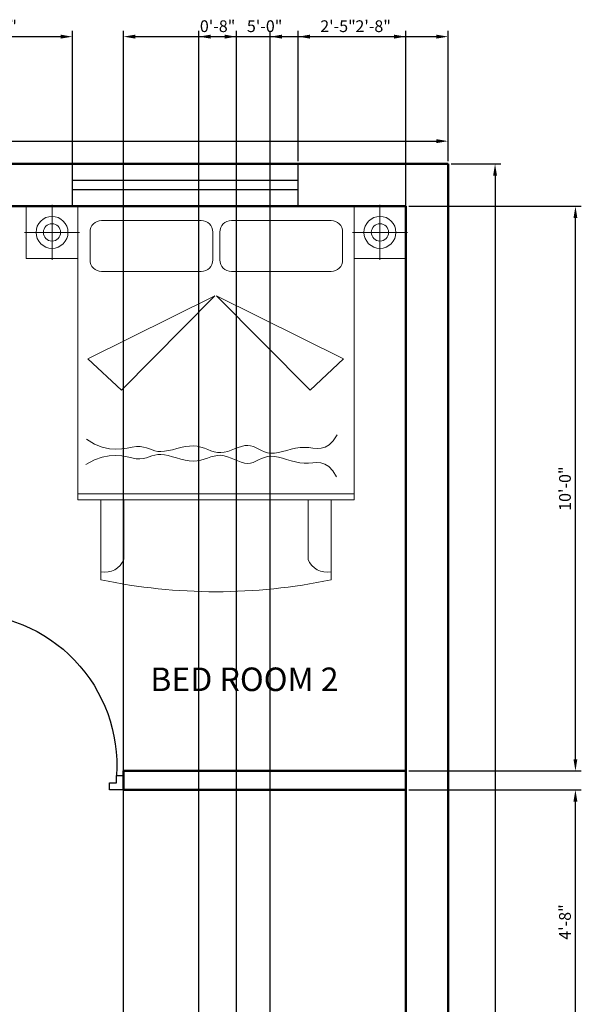
# Model space of a CAD drawing. Units: inches. Extents: x 1905 to 2315, y 3232 to 3824.
# Tile 8 of 8: x 2195 to 2314, y 3615 to 3824. Entities that reach past the tile are written whole.
import ezdxf

# ---------------------------------------------------------------- set-up
doc = ezdxf.new("R2010")
doc.units = ezdxf.units.IN
for name, color, linetype, lineweight in [('A-ANNO-DIMS', 2, 'Continuous', 18), ('A-AREA-IDEN', 7, 'Continuous', 25), ('A-FURN', 8, 'Continuous', 18), ('door', 1, 'Continuous', 25), ('wall', 2, 'Continuous', 50), ('WINDOW', 60, 'Continuous', 25)]:
    doc.layers.add(name, color=color, linetype=linetype, lineweight=lineweight)
doc.styles.get("Standard").update_dxf_attribs({"font": 'arial.ttf'})
doc.dimstyles.new('ISO-25', dxfattribs={"dimtxt": 2.5, "dimasz": 2.5, "dimexe": 1.25, "dimexo": 0.625, "dimtad": 1, "dimdec": 1, "dimlunit": 3, "dimtxsty": 'Standard', "dimcen": 2.5, "dimadec": 0, "dimazin": 0, "dimtfac": 1, "dimtdec": 1, "dimtmove": 0, "dimatfit": 3, "dimfxl": 1, "dimarcsym": 0})

# ---------------------------------------------------------------- blocks, each defined once
blk = doc.blocks.new('A$C4F543DC7')
for p, q in [((0.0134, 3.35, -0.1688), (3.3134, 3.35, -0.1688)), ((0.4634, 3.35, -0.1688), (0.0134, 3.35, -0.1688)), ((0.0134, 2.896, -0.1688), (0.0134, 3.35, -0.1688)), ((0.0134, 3.35, -0.1688), (0.0134, 2.896, -0.1688)), ((0.2381, 3.1233, -0.4388), (0.2381, 3.3614, -0.4388)), ((0.4634, 3.35, -0.1688), (0.4634, 0.8, -0.1688)), ((2.8634, 3.35, -0.1688), (0.4634, 3.35, -0.1688)), ((0.4634, 2.896, -0.1688), (0.4634, 3.35, -0.1688)), ((2.8634, 0.8, -0.1688), (2.8634, 3.35, -0.1688)), ((2.8634, 3.35, -0.1688), (3.3134, 3.35, -0.1688)), ((2.8634, 2.896, -0.1688), (2.8634, 3.35, -0.1688)), ((3.0888, 3.1233, -0.4388), (3.0888, 3.3614, -0.4388)), ((3.3134, 3.35, -0.1688), (3.3134, 2.896, -0.1688)), ((3.3134, 3.35, -0.1688), (3.3134, 2.896, -0.1688)), ((1.5354, 3.226, -0.1688), (0.6684, 3.226, -0.1688)), ((2.6644, 3.226, -0.1688), (1.7974, 3.226, -0.1688)), ((0.2381, 3.1233, -0.4388), (0, 3.1233, -0.4388)), ((0.2381, 3.1233, -0.4388), (0.4762, 3.1233, -0.4388)), ((0.2381, 3.1233, -0.4388), (0.2381, 2.8852, -0.4388)), ((0.5684, 3.126, -0.1688), (0.5684, 2.884, -0.1688)), ((1.6354, 2.884, -0.1688), (1.6354, 3.126, -0.1688)), ((1.6974, 3.126, -0.1688), (1.6974, 2.884, -0.1688)), ((2.7644, 2.884, -0.1688), (2.7644, 3.126, -0.1688)), ((3.0888, 3.1233, -0.4388), (2.8507, 3.1233, -0.4388)), ((3.0888, 3.1233, -0.4388), (3.0888, 2.8852, -0.4388)), ((3.0888, 3.1233, -0.4388), (3.3269, 3.1233, -0.4388)), ((0.4634, 2.896, -0.1688), (0.0134, 2.896, -0.1688)), ((0.0134, 2.896, -0.1688), (0.4634, 2.896, -0.1688)), ((0.4634, 0.8, -0.1688), (0.4634, 2.896, -0.1688)), ((2.8634, 2.896, -0.1688), (2.8634, 0.8, -0.1688)), ((3.3134, 2.896, -0.1688), (2.8634, 2.896, -0.1688)), ((3.3134, 2.896, -0.1688), (2.8634, 2.896, -0.1688)), ((0.6684, 2.784, -0.1688), (1.5354, 2.784, -0.1688)), ((1.7974, 2.784, -0.1688), (2.6644, 2.784, -0.1688)), ((1.6534, 2.573, -0.1688), (0.5504, 2.025, -0.1688)), ((0.8414, 1.752, -0.1688), (1.6534, 2.573, -0.1688)), ((2.4814, 1.752, -0.1688), (1.6694, 2.573, -0.1688)), ((1.6694, 2.573, -0.1688), (2.7724, 2.025, -0.1688)), ((0.5504, 2.025, -0.1688), (0.8414, 1.752, -0.1688)), ((2.7724, 2.025, -0.1688), (2.4814, 1.752, -0.1688)), ((0.5369, 1.3267, -0.1688), (0.6088, 1.2835, -0.1688)), ((2.6479, 1.2774, -0.1688), (2.683, 1.312, -0.1688)), ((2.683, 1.312, -0.1688), (2.7182, 1.3641, -0.1688)), ((0.6088, 1.2835, -0.1688), (0.6756, 1.2566, -0.1688)), ((0.6756, 1.2566, -0.1688), (0.7373, 1.2428, -0.1688)), ((0.7373, 1.2428, -0.1688), (0.794, 1.239, -0.1688)), ((0.794, 1.239, -0.1688), (0.8457, 1.242, -0.1688)), ((0.8457, 1.242, -0.1688), (0.8925, 1.2489, -0.1688)), ((0.8925, 1.2489, -0.1688), (0.9345, 1.2564, -0.1688)), ((0.9345, 1.2564, -0.1688), (0.9718, 1.2615, -0.1688)), ((0.9718, 1.2615, -0.1688), (1.0044, 1.2617, -0.1688)), ((1.0044, 1.2617, -0.1688), (1.0334, 1.2578, -0.1688)), ((1.0334, 1.2578, -0.1688), (1.0597, 1.2509, -0.1688)), ((1.0597, 1.2509, -0.1688), (1.0842, 1.2424, -0.1688)), ((1.0842, 1.2424, -0.1688), (1.1081, 1.2336, -0.1688)), ((1.1081, 1.2336, -0.1688), (1.1322, 1.2257, -0.1688)), ((1.1322, 1.2257, -0.1688), (1.1577, 1.2201, -0.1688)), ((1.1577, 1.2201, -0.1688), (1.1855, 1.218, -0.1688)), ((1.1855, 1.218, -0.1688), (1.2163, 1.2204, -0.1688)), ((1.2163, 1.2204, -0.1688), (1.2498, 1.2264, -0.1688)), ((1.2498, 1.2264, -0.1688), (1.2852, 1.2347, -0.1688)), ((1.2852, 1.2347, -0.1688), (1.3218, 1.2441, -0.1688)), ((1.3218, 1.2441, -0.1688), (1.3591, 1.2533, -0.1688)), ((1.3591, 1.2533, -0.1688), (1.3963, 1.2612, -0.1688)), ((1.3963, 1.2612, -0.1688), (1.4328, 1.2664, -0.1688)), ((1.4328, 1.2664, -0.1688), (1.4679, 1.2677, -0.1688)), ((1.4679, 1.2677, -0.1688), (1.501, 1.2643, -0.1688)), ((1.501, 1.2643, -0.1688), (1.5324, 1.257, -0.1688)), ((1.5324, 1.257, -0.1688), (1.5624, 1.2473, -0.1688)), ((1.5624, 1.2473, -0.1688), (1.5915, 1.2365, -0.1688)), ((1.5915, 1.2365, -0.1688), (1.6199, 1.2259, -0.1688)), ((1.6199, 1.2259, -0.1688), (1.6481, 1.2169, -0.1688)), ((1.6481, 1.2169, -0.1688), (1.6765, 1.2108, -0.1688)), ((1.6765, 1.2108, -0.1688), (1.7053, 1.209, -0.1688)), ((1.7053, 1.209, -0.1688), (1.7349, 1.2124, -0.1688)), ((1.7349, 1.2124, -0.1688), (1.7651, 1.2199, -0.1688)), ((1.7651, 1.2199, -0.1688), (1.7955, 1.2301, -0.1688)), ((1.7955, 1.2301, -0.1688), (1.8258, 1.2417, -0.1688)), ((1.8258, 1.2417, -0.1688), (1.8557, 1.2531, -0.1688)), ((1.8557, 1.2531, -0.1688), (1.8849, 1.263, -0.1688)), ((1.8849, 1.263, -0.1688), (1.913, 1.2698, -0.1688)), ((1.913, 1.2698, -0.1688), (1.9397, 1.2722, -0.1688)), ((1.9397, 1.2722, -0.1688), (1.9649, 1.2692, -0.1688)), ((1.9649, 1.2692, -0.1688), (1.989, 1.2617, -0.1688)), ((1.989, 1.2617, -0.1688), (2.0124, 1.2512, -0.1688)), ((2.0124, 1.2512, -0.1688), (2.0359, 1.2391, -0.1688)), ((2.0359, 1.2391, -0.1688), (2.0599, 1.2269, -0.1688)), ((2.0599, 1.2269, -0.1688), (2.0849, 1.216, -0.1688)), ((2.0849, 1.216, -0.1688), (2.1117, 1.2077, -0.1688)), ((2.1117, 1.2077, -0.1688), (2.1407, 1.2037, -0.1688)), ((2.1407, 1.2037, -0.1688), (2.1723, 1.2047, -0.1688)), ((2.1723, 1.2047, -0.1688), (2.2062, 1.21, -0.1688)), ((2.2062, 1.21, -0.1688), (2.242, 1.2182, -0.1688)), ((2.242, 1.2182, -0.1688), (2.2791, 1.2279, -0.1688)), ((2.2791, 1.2279, -0.1688), (2.3173, 1.2378, -0.1688)), ((2.3173, 1.2378, -0.1688), (2.3558, 1.2465, -0.1688)), ((2.3558, 1.2465, -0.1688), (2.3944, 1.2527, -0.1688)), ((2.3944, 1.2527, -0.1688), (2.4325, 1.255, -0.1688)), ((2.4325, 1.255, -0.1688), (2.4698, 1.2529, -0.1688)), ((2.4698, 1.2529, -0.1688), (2.5064, 1.2488, -0.1688)), ((2.5064, 1.2488, -0.1688), (2.5423, 1.2459, -0.1688)), ((2.5423, 1.2459, -0.1688), (2.5777, 1.2476, -0.1688)), ((2.5777, 1.2476, -0.1688), (2.6129, 1.257, -0.1688)), ((2.6129, 1.257, -0.1688), (2.6479, 1.2774, -0.1688)), ((0.5334, 1.105, -0.1688), (0.6067, 1.1458, -0.1688)), ((0.6067, 1.1458, -0.1688), (0.6743, 1.1706, -0.1688)), ((0.6743, 1.1706, -0.1688), (0.7364, 1.1825, -0.1688)), ((0.7364, 1.1825, -0.1688), (0.7931, 1.1846, -0.1688)), ((0.7931, 1.1846, -0.1688), (0.8447, 1.1799, -0.1688)), ((0.8447, 1.1799, -0.1688), (0.8913, 1.1716, -0.1688)), ((0.8913, 1.1716, -0.1688), (0.9331, 1.1628, -0.1688)), ((0.9331, 1.1628, -0.1688), (0.9701, 1.1565, -0.1688)), ((0.9701, 1.1565, -0.1688), (1.0027, 1.1552, -0.1688)), ((1.0027, 1.1552, -0.1688), (1.0318, 1.1582, -0.1688)), ((1.0318, 1.1582, -0.1688), (1.0583, 1.1642, -0.1688)), ((1.0583, 1.1642, -0.1688), (1.0831, 1.172, -0.1688)), ((1.0831, 1.172, -0.1688), (1.1072, 1.18, -0.1688)), ((1.1072, 1.18, -0.1688), (1.1316, 1.1872, -0.1688)), ((1.1316, 1.1872, -0.1688), (1.1573, 1.192, -0.1688)), ((1.1573, 1.192, -0.1688), (1.1851, 1.1932, -0.1688)), ((1.1851, 1.1932, -0.1688), (1.2158, 1.1898, -0.1688)), ((1.2158, 1.1898, -0.1688), (1.2491, 1.1828, -0.1688)), ((1.2491, 1.1828, -0.1688), (1.2842, 1.1734, -0.1688)), ((1.2842, 1.1734, -0.1688), (1.3206, 1.1629, -0.1688)), ((1.3206, 1.1629, -0.1688), (1.3575, 1.1524, -0.1688)), ((1.3575, 1.1524, -0.1688), (1.3945, 1.1434, -0.1688)), ((1.3945, 1.1434, -0.1688), (1.4308, 1.1371, -0.1688)), ((1.4308, 1.1371, -0.1688), (1.4658, 1.1347, -0.1688)), ((1.4658, 1.1347, -0.1688), (1.499, 1.137, -0.1688)), ((1.499, 1.137, -0.1688), (1.5306, 1.1433, -0.1688)), ((1.5306, 1.1433, -0.1688), (1.5609, 1.152, -0.1688)), ((1.5609, 1.152, -0.1688), (1.5903, 1.1619, -0.1688)), ((1.5903, 1.1619, -0.1688), (1.6191, 1.1716, -0.1688)), ((1.6191, 1.1716, -0.1688), (1.6475, 1.1797, -0.1688)), ((1.6475, 1.1797, -0.1688), (1.676, 1.1849, -0.1688)), ((1.676, 1.1849, -0.1688), (1.7049, 1.1858, -0.1688)), ((1.7049, 1.1858, -0.1688), (1.7344, 1.1816, -0.1688)), ((1.7344, 1.1816, -0.1688), (1.7643, 1.1731, -0.1688)), ((1.7643, 1.1731, -0.1688), (1.7944, 1.1619, -0.1688)), ((1.7944, 1.1619, -0.1688), (1.8244, 1.1494, -0.1688)), ((1.8244, 1.1494, -0.1688), (1.8539, 1.137, -0.1688)), ((1.8539, 1.137, -0.1688), (1.8827, 1.1263, -0.1688)), ((1.8827, 1.1263, -0.1688), (1.9106, 1.1186, -0.1688)), ((1.9106, 1.1186, -0.1688), (1.9373, 1.1153, -0.1688)), ((1.9373, 1.1153, -0.1688), (1.9625, 1.1176, -0.1688)), ((1.9625, 1.1176, -0.1688), (1.9868, 1.1243, -0.1688)), ((1.9868, 1.1243, -0.1688), (2.0106, 1.134, -0.1688)), ((2.0106, 1.134, -0.1688), (2.0344, 1.1454, -0.1688)), ((2.0344, 1.1454, -0.1688), (2.0588, 1.1568, -0.1688)), ((2.0588, 1.1568, -0.1688), (2.0842, 1.167, -0.1688)), ((2.0842, 1.167, -0.1688), (2.1112, 1.1743, -0.1688)), ((2.1112, 1.1743, -0.1688), (2.1403, 1.1775, -0.1688)), ((2.1403, 1.1775, -0.1688), (2.1718, 1.1755, -0.1688)), ((2.1718, 1.1755, -0.1688), (2.2056, 1.1691, -0.1688)), ((2.2056, 1.1691, -0.1688), (2.2411, 1.1598, -0.1688)), ((2.2411, 1.1598, -0.1688), (2.2779, 1.1489, -0.1688)), ((2.2779, 1.1489, -0.1688), (2.3157, 1.1379, -0.1688)), ((2.3157, 1.1379, -0.1688), (2.354, 1.1279, -0.1688)), ((2.354, 1.1279, -0.1688), (2.3923, 1.1205, -0.1688)), ((2.3923, 1.1205, -0.1688), (2.4304, 1.117, -0.1688)), ((2.4304, 1.117, -0.1688), (2.4677, 1.118, -0.1688)), ((2.4677, 1.118, -0.1688), (2.5043, 1.1209, -0.1688)), ((2.5043, 1.1209, -0.1688), (2.5403, 1.1226, -0.1688)), ((2.5403, 1.1226, -0.1688), (2.5757, 1.1199, -0.1688)), ((2.5757, 1.1199, -0.1688), (2.6106, 1.1094, -0.1688)), ((2.6106, 1.1094, -0.1688), (2.645, 1.0879, -0.1688)), ((2.645, 1.0879, -0.1688), (2.6789, 1.0522, -0.1688)), ((2.6789, 1.0522, -0.1688), (2.7124, 0.999, -0.1688)), ((0.4634, 0.85, -0.1688), (2.8634, 0.85, -0.1688)), ((0.4634, 0.8, -0.1688), (2.8634, 0.8, -0.1688)), ((0.6634, 0.8, -0.1688), (0.4634, 0.8, -0.1688)), ((0.6634, 0.8, -0.1688), (2.6634, 0.8, -0.1688)), ((0.6634, 0.104, -0.1688), (0.6634, 0.8, -0.1688)), ((0.6634, 0.104, -0.1688), (0.6634, 0.8, -0.1688)), ((0.8634, 0.281, -0.1688), (0.8634, 0.8, -0.1688)), ((2.4634, 0.8, -0.1688), (2.4634, 0.281, -0.1688)), ((2.8634, 0.8, -0.1688), (2.6634, 0.8, -0.1688)), ((2.6634, 0.8, -0.1688), (2.6634, 0.104, -0.1688)), ((2.6634, 0.8, -0.1688), (2.6634, 0.104, -0.1688))]:
    blk.add_line(p, q)
for centre, radius in [((0.2381, 3.1233, -0.4388), 0.139), ((3.0888, 3.1233, -0.4388), 0.139), ((0.2381, 3.1233, -0.4388), 0.075), ((3.0888, 3.1233, -0.4388), 0.075)]:
    blk.add_circle(centre, radius)
for centre, radius, start, end in [((0.6684, 3.126, -0.1688), 0.1, 90, 180), ((1.5354, 3.126, -0.1688), 0.1, 0, 90), ((1.7974, 3.126, -0.1688), 0.1, 90, 180), ((2.6644, 3.126, -0.1688), 0.1, 0, 90), ((0.6684, 2.884, -0.1688), 0.1, 180, 270), ((1.5354, 2.884, -0.1688), 0.1, 270, 0), ((1.7974, 2.884, -0.1688), 0.1, 180, 270), ((2.6644, 2.884, -0.1688), 0.1, 270, 0), ((0.6994, 0.3472, -0.1688), 0.1769, 258.2616, 338.03196), ((2.6275, 0.3472, -0.1688), 0.1769, 201.96804, 281.7384), ((1.6634, 4.8597, -0.1688), 4.8597, 258.12517, 281.87483), ((1.6634, 4.8597, -0.1688), 4.8597, 258.12517, 281.87483)]:
    blk.add_arc(centre, radius, start, end)
blk = doc.blocks.new('*D15')
at = {"layer": 'A-ANNO-DIMS', "color": 0, "lineweight": -2, "transparency": 16777216}
for p, q in [((1938.01, 3793.86), (1938.01, 3799.33)), ((2286.01, 3793.86), (2286.01, 3799.33)), ((1940.51, 3798.08), (2283.51, 3798.08))]:
    blk.add_line(p, q, dxfattribs=at)
at = {"layer": 'A-ANNO-DIMS', "color": 0, "transparency": 16777216}
for points in [[(1940.51, 3798.5), (1940.51, 3797.67), (1938.01, 3798.08)], [(2283.51, 3798.5), (2283.51, 3797.67), (2286.01, 3798.08)]]:
    blk.add_solid(points, dxfattribs=at)
at = {"layer": 'Defpoints', "color": 0, "transparency": 16777216}
for p in [(2286.01, 3798.08), (1938.01, 3793.23), (2286.01, 3793.23)]:
    blk.add_point(p, dxfattribs=at)
at = {"layer": 'A-ANNO-DIMS', "color": 0, "transparency": 16777216, "insert": (2112.01, 3799.99), "char_height": 2.5, "attachment_point": 5}
blk.add_mtext("29'", dxfattribs=at)
blk = doc.blocks.new('*D16')
at = {"layer": 'A-ANNO-DIMS', "color": 0, "lineweight": -2, "transparency": 16777216}
for p, q in [((2286.63, 3793.23), (2297.23, 3793.23)), ((2295.98, 3790.73), (2295.98, 3279.73)), ((2286.63, 3277.23), (2297.23, 3277.23))]:
    blk.add_line(p, q, dxfattribs=at)
at = {"layer": 'A-ANNO-DIMS', "color": 0, "transparency": 16777216}
for points in [[(2295.57, 3790.73), (2296.4, 3790.73), (2295.98, 3793.23)], [(2295.57, 3279.73), (2296.4, 3279.73), (2295.98, 3277.23)]]:
    blk.add_solid(points, dxfattribs=at)
at = {"layer": 'Defpoints', "color": 0, "transparency": 16777216}
for p in [(2286.01, 3793.23), (2286.01, 3277.23), (2295.98, 3277.23)]:
    blk.add_point(p, dxfattribs=at)
at = {"layer": 'A-ANNO-DIMS', "color": 0, "transparency": 16777216, "insert": (2294.08, 3535.23), "char_height": 2.5, "attachment_point": 5, "rotation": 90}
blk.add_mtext("43'", dxfattribs=at)
blk = doc.blocks.new('DOOR-SWING-36IN')
for p, q in [((34.51, 36), (37.51, 36)), ((34.51, 34.5), (34.51, 36)), ((37.51, 36), (37.51, 33)), ((36.01, 34.5), (0.01, 34.5)), ((36.01, 34.5), (34.51, 34.5)), ((36.01, 33), (36.01, 34.5)), ((36.01, 33), (0.01, 33)), ((37.51, 33), (36.01, 33)), ((37.51, 3), (36.01, 3)), ((36.01, 3), (36.01, 1.5)), ((37.51, 0), (37.51, 3)), ((36.01, 1.5), (34.51, 1.5)), ((34.51, 1.5), (34.51, 0)), ((34.51, 0), (37.51, 0))]:
    blk.add_line(p, q)
blk.add_arc((32.32, 33.75), 32.32, 178.6705, 273.8756)
blk = doc.blocks.new('WIN-48IN')
for p, q in [((0, 9), (0, 0)), ((0, 9), (48, 9)), ((48, 9), (48, 0)), ((0, 5.5), (48, 5.5)), ((0, 3.5), (48, 3.5)), ((0, 0), (48, 0))]:
    blk.add_line(p, q)
blk = doc.blocks.new('*D42')
at = {"layer": 'A-ANNO-DIMS', "color": 0, "lineweight": -2, "transparency": 16777216}
for p, q in [((2175.01, 3784.86), (2175.01, 3821.54)), ((2206.15, 3784.86), (2206.15, 3821.54)), ((2177.51, 3820.29), (2203.65, 3820.29))]:
    blk.add_line(p, q, dxfattribs=at)
at = {"layer": 'A-ANNO-DIMS', "color": 0, "transparency": 16777216}
for points in [[(2177.51, 3820.71), (2177.51, 3819.88), (2175.01, 3820.29)], [(2203.65, 3820.71), (2203.65, 3819.88), (2206.15, 3820.29)]]:
    blk.add_solid(points, dxfattribs=at)
at = {"layer": 'Defpoints', "color": 0, "transparency": 16777216}
for p in [(2206.15, 3820.29), (2175.01, 3784.23), (2206.15, 3784.23)]:
    blk.add_point(p, dxfattribs=at)
at = {"layer": 'A-ANNO-DIMS', "color": 0, "transparency": 16777216, "insert": (2190.58, 3822.17), "char_height": 2.5, "attachment_point": 5}
blk.add_mtext('2\'-7"', dxfattribs=at)
blk = doc.blocks.new('*D43')
at = {"layer": 'A-ANNO-DIMS', "color": 0, "lineweight": -2, "transparency": 16777216}
for p, q in [((2254.15, 3793.86), (2254.15, 3821.54)), ((2286.01, 3793.86), (2286.01, 3821.54)), ((2256.65, 3820.29), (2283.51, 3820.29))]:
    blk.add_line(p, q, dxfattribs=at)
at = {"layer": 'A-ANNO-DIMS', "color": 0, "transparency": 16777216}
for points in [[(2256.65, 3820.71), (2256.65, 3819.88), (2254.15, 3820.29)], [(2283.51, 3820.71), (2283.51, 3819.88), (2286.01, 3820.29)]]:
    blk.add_solid(points, dxfattribs=at)
at = {"layer": 'Defpoints', "color": 0, "transparency": 16777216}
for p in [(2286.01, 3820.29), (2254.15, 3793.23), (2286.01, 3793.23)]:
    blk.add_point(p, dxfattribs=at)
at = {"layer": 'A-ANNO-DIMS', "color": 0, "transparency": 16777216, "insert": (2270.08, 3822.19), "char_height": 2.5, "attachment_point": 5}
blk.add_mtext('2\'-8"', dxfattribs=at)
blk = doc.blocks.new('*D54')
at = {"layer": 'A-ANNO-DIMS', "color": 0, "lineweight": -2, "transparency": 16777216}
for p, q in [((2277.63, 3660.23), (2314.32, 3660.23)), ((2313.07, 3606.51), (2313.07, 3657.73)), ((2277.63, 3604.01), (2314.32, 3604.01))]:
    blk.add_line(p, q, dxfattribs=at)
at = {"layer": 'A-ANNO-DIMS', "color": 0, "transparency": 16777216}
for points in [[(2312.65, 3657.73), (2313.48, 3657.73), (2313.07, 3660.23)], [(2312.65, 3606.51), (2313.48, 3606.51), (2313.07, 3604.01)]]:
    blk.add_solid(points, dxfattribs=at)
at = {"layer": 'Defpoints', "color": 0, "transparency": 16777216}
for p in [(2277.01, 3660.23), (2313.07, 3660.23), (2277.01, 3604.01)]:
    blk.add_point(p, dxfattribs=at)
at = {"layer": 'A-ANNO-DIMS', "color": 0, "transparency": 16777216, "insert": (2311.17, 3632.12), "char_height": 2.5, "attachment_point": 5, "rotation": 90}
blk.add_mtext('4\'-8"', dxfattribs=at)
blk = doc.blocks.new('*D55')
at = {"layer": 'A-ANNO-DIMS', "color": 0, "lineweight": -2, "transparency": 16777216}
for p, q in [((2277.63, 3784.23), (2314.32, 3784.23)), ((2313.07, 3666.73), (2313.07, 3781.73)), ((2277.63, 3664.23), (2314.32, 3664.23))]:
    blk.add_line(p, q, dxfattribs=at)
at = {"layer": 'A-ANNO-DIMS', "color": 0, "transparency": 16777216}
for points in [[(2312.65, 3781.73), (2313.48, 3781.73), (2313.07, 3784.23)], [(2312.65, 3666.73), (2313.48, 3666.73), (2313.07, 3664.23)]]:
    blk.add_solid(points, dxfattribs=at)
at = {"layer": 'Defpoints', "color": 0, "transparency": 16777216}
for p in [(2277.01, 3784.23), (2313.07, 3784.23), (2277.01, 3664.23)]:
    blk.add_point(p, dxfattribs=at)
at = {"layer": 'A-ANNO-DIMS', "color": 0, "transparency": 16777216, "insert": (2311.17, 3724.23), "char_height": 2.5, "attachment_point": 5, "rotation": 90}
blk.add_mtext('10\'-0"', dxfattribs=at)
blk = doc.blocks.new('*D62')
at = {"layer": 'A-ANNO-DIMS', "color": 0, "lineweight": -2, "transparency": 16777216}
for p, q in [((2233.01, 3322.86), (2233.01, 3821.54)), ((2241.01, 3322.86), (2241.01, 3821.54)), ((2235.51, 3820.29), (2238.51, 3820.29))]:
    blk.add_line(p, q, dxfattribs=at)
at = {"layer": 'A-ANNO-DIMS', "color": 0, "transparency": 16777216}
for points in [[(2235.51, 3820.71), (2235.51, 3819.88), (2233.01, 3820.29)], [(2238.51, 3820.71), (2238.51, 3819.88), (2241.01, 3820.29)]]:
    blk.add_solid(points, dxfattribs=at)
at = {"layer": 'Defpoints', "color": 0, "transparency": 16777216}
for p in [(2241.01, 3820.29), (2233.01, 3322.23), (2241.01, 3322.23)]:
    blk.add_point(p, dxfattribs=at)
at = {"layer": 'A-ANNO-DIMS', "color": 0, "transparency": 16777216, "insert": (2237.01, 3822.19), "char_height": 2.5, "attachment_point": 5}
blk.add_mtext('0\'-8"', dxfattribs=at)
blk = doc.blocks.new('*D66')
at = {"layer": 'A-ANNO-DIMS', "color": 0, "lineweight": -2, "transparency": 16777216}
for p, q in [((2248.2, 3393.73), (2248.2, 3821.54)), ((2277.01, 3383.48), (2277.01, 3821.54)), ((2250.7, 3820.29), (2274.51, 3820.29))]:
    blk.add_line(p, q, dxfattribs=at)
at = {"layer": 'A-ANNO-DIMS', "color": 0, "transparency": 16777216}
for points in [[(2250.7, 3820.71), (2250.7, 3819.88), (2248.2, 3820.29)], [(2274.51, 3820.71), (2274.51, 3819.88), (2277.01, 3820.29)]]:
    blk.add_solid(points, dxfattribs=at)
at = {"layer": 'Defpoints', "color": 0, "transparency": 16777216}
for p in [(2277.01, 3820.29), (2248.2, 3393.11), (2277.01, 3382.85)]:
    blk.add_point(p, dxfattribs=at)
at = {"layer": 'A-ANNO-DIMS', "color": 0, "transparency": 16777216, "insert": (2262.6, 3822.19), "char_height": 2.5, "attachment_point": 5}
blk.add_mtext('2\'-5"', dxfattribs=at)
blk = doc.blocks.new('*D71')
at = {"layer": 'A-ANNO-DIMS', "color": 0, "lineweight": -2, "transparency": 16777216}
for p, q in [((2217.01, 3480.07), (2217.01, 3821.54)), ((2277.01, 3476.07), (2277.01, 3821.54)), ((2219.51, 3820.29), (2274.51, 3820.29))]:
    blk.add_line(p, q, dxfattribs=at)
at = {"layer": 'A-ANNO-DIMS', "color": 0, "transparency": 16777216}
for points in [[(2219.51, 3820.71), (2219.51, 3819.88), (2217.01, 3820.29)], [(2274.51, 3820.71), (2274.51, 3819.88), (2277.01, 3820.29)]]:
    blk.add_solid(points, dxfattribs=at)
at = {"layer": 'Defpoints', "color": 0, "transparency": 16777216}
for p in [(2277.01, 3820.29), (2217.01, 3479.45), (2277.01, 3475.45)]:
    blk.add_point(p, dxfattribs=at)
at = {"layer": 'A-ANNO-DIMS', "color": 0, "transparency": 16777216, "insert": (2247.01, 3822.19), "char_height": 2.5, "attachment_point": 5}
blk.add_mtext('5\'-0"', dxfattribs=at)

msp = doc.modelspace()

# ---------------------------------------------------------------- linework, layer by layer
at = {"layer": 'wall'}
for p, q in [((2286.01, 3793.23), (1938.01, 3793.23)), ((2286.01, 3277.23), (2286.01, 3793.23)), ((2277.01, 3784.23), (1947.01, 3784.23)), ((2277.01, 3286.23), (2277.01, 3784.23)), ((2277.01, 3664.23), (2217.01, 3664.23)), ((2217.01, 3664.23), (2217.01, 3660.23)), ((2277.01, 3660.23), (2217.01, 3660.23))]:
    msp.add_line(p, q, dxfattribs=at)

# ---------------------------------------------------------------- block references
at = {"layer": 'A-FURN', "xscale": 24.45263891714, "yscale": 24.45263891714, "zscale": 24.45263891714}
msp.add_blockref('A$C4F543DC7', (2195.99, 3702.32, 4.13), dxfattribs=at)
at = {"layer": 'door', "extrusion": (0, 0, -1), "zscale": -1, "rotation": 270.0000000000044}
msp.add_blockref('DOOR-SWING-36IN', (-2217.01, 3697.74), dxfattribs=at)
at = {"layer": 'WINDOW', "rotation": 180}
msp.add_blockref('WIN-48IN', (2254.15, 3793.23), dxfattribs=at)

# ---------------------------------------------------------------- texts
at = {"layer": 'A-AREA-IDEN', "insert": (2222.7, 3686.21), "char_height": 5, "attachment_point": 1}
msp.add_mtext_dynamic_manual_height_columns('BED ROOM 2', width=56.1502, gutter_width=12.5, heights=[0], dxfattribs=at)

# ---------------------------------------------------------------- dimensions: what is measured, and where the dimension line sits
at = {"layer": 'A-ANNO-DIMS'}
for base, p1, p2, override, picture, middle in [((2206.15, 3820.29), (2175.01, 3784.23), (2206.15, 3784.23), {"dimdec": 1, "dimlfac": 1, "dimrnd": 0, "dimzin": 1, "dimdsep": 46, "dimlunit": 4, "dimfrac": 2}, '*D42', (2190.58, 3822.17)), ((2277.01, 3820.29), (2217.01, 3479.45), (2277.01, 3475.45), {"dimdec": 1, "dimlfac": 1, "dimrnd": 0, "dimzin": 1, "dimdsep": 46, "dimlunit": 4, "dimfrac": 2}, '*D71', (2247.01, 3822.19)), ((2241.01, 3820.29), (2233.01, 3322.23), (2241.01, 3322.23), {"dimdec": 1, "dimlfac": 1, "dimrnd": 0, "dimzin": 1, "dimdsep": 46, "dimlunit": 4, "dimfrac": 2}, '*D62', (2237.01, 3822.19)), ((2277.01, 3820.29), (2248.2, 3393.11), (2277.01, 3382.85), {"dimdec": 1, "dimlfac": 1, "dimrnd": 0, "dimzin": 1, "dimdsep": 46, "dimlunit": 4, "dimfrac": 2}, '*D66', (2262.6, 3822.19)), ((2286.01, 3820.29), (2254.15, 3793.23), (2286.01, 3793.23), {"dimdec": 1, "dimlfac": 1, "dimrnd": 0, "dimzin": 1, "dimdsep": 46, "dimlunit": 4, "dimfrac": 2}, '*D43', (2270.08, 3822.19)), ((2286.01, 3798.08), (1938.01, 3793.23), (2286.01, 3793.23), {"dimclrd": 0, "dimclre": 0, "dimclrt": 0}, '*D15', (2112.01, 3799.99))]:
    dim = msp.add_linear_dim(base=base, p1=p1, p2=p2, dimstyle='ISO-25', override=override, dxfattribs=at)
    dim.commit()
    dim.dimension.update_dxf_attribs({"geometry": picture, "text_midpoint": middle})
for base, p1, p2, override, picture, middle in [((2295.98, 3277.23), (2286.01, 3793.23), (2286.01, 3277.23), {"dimclrd": 0, "dimclre": 0, "dimclrt": 0}, '*D16', (2294.08, 3535.23)), ((2313.07, 3784.23), (2277.01, 3664.23), (2277.01, 3784.23), {"dimdec": 1, "dimlfac": 1, "dimrnd": 0, "dimzin": 1, "dimdsep": 46, "dimlunit": 4, "dimfrac": 2}, '*D55', (2311.17, 3724.23)), ((2313.07, 3660.23), (2277.01, 3604.01), (2277.01, 3660.23), {"dimdec": 1, "dimlfac": 1, "dimrnd": 0, "dimzin": 1, "dimdsep": 46, "dimlunit": 4, "dimfrac": 2}, '*D54', (2311.17, 3632.12))]:
    dim = msp.add_linear_dim(base=base, p1=p1, p2=p2, angle=90, dimstyle='ISO-25', override=override, dxfattribs=at)
    dim.commit()
    dim.dimension.update_dxf_attribs({"geometry": picture, "text_midpoint": middle})

doc.saveas('drawing.dxf')
